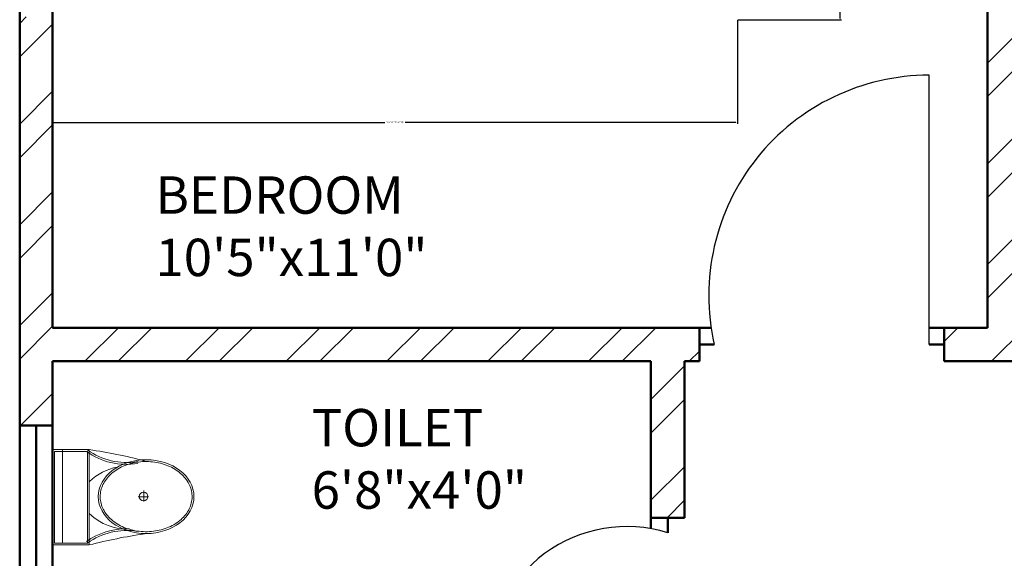
# Model space of a CAD drawing. Units: inches. Extents: x 1901 to 2863, y 888 to 2433.
# Tile 15 of 91: x 2025 to 2157, y 1549 to 1621. Entities that reach past the tile are written whole.
import ezdxf

# ---------------------------------------------------------------- set-up
doc = ezdxf.new("R2010")
doc.units = ezdxf.units.IN
for name, color, linetype, lineweight in [('A-ANNO-DIMS', 2, 'Continuous', 18), ('A-AREA-IDEN', 7, 'Continuous', 18), ('A-DOOR', 4, 'Continuous', 25), ('A-FLOR-FIXT', 9, 'Continuous', 18), ('A-WALL', 7, 'Continuous', 50), ('A-WALL-PATT', 8, 'Continuous', 13)]:
    doc.layers.add(name, color=color, linetype=linetype, lineweight=lineweight)
doc.styles.get("Standard").update_dxf_attribs({"font": 'arial.ttf'})
doc.dimstyles.get("Standard").update_dxf_attribs({"dimtxt": 0.18, "dimasz": 0.18, "dimexe": 0.18, "dimexo": 0.0625, "dimgap": 0.09, "dimtad": 0, "dimtih": 1, "dimtoh": 1, "dimdec": 4, "dimzin": 0, "dimdsep": 46, "dimtxsty": 'Standard', "dimcen": 0.09, "dimadec": 0, "dimazin": 0, "dimtfac": 1, "dimtdec": 4, "dimtofl": 0, "dimtmove": 0, "dimatfit": 3, "dimfxl": 1, "dimtolj": 1, "dimtzin": 0, "dimarcsym": 0})

# ---------------------------------------------------------------- blocks, each defined once
blk = doc.blocks.new('A$C31115884')
for p, q in [((283.1, 497.7), (223.4, 497.7)), ((257.5, 466.4), (257.5, 523.2)), ((0, 200), (0, 0)), ((520, 200), (0, 200)), ((10, 190), (10, 10)), ((510, 190), (10, 190)), ((510, 10), (510, 190)), ((520, 0), (520, 200)), ((510, 54.5), (0, 54.5)), ((10, 10), (510, 10)), ((0, 0), (520, 0))]:
    blk.add_line(p, q)
blk.add_circle((255.6, 496.4), 23.6)
for centre, radius, start, end in [((2777.7, -204.6), 2807, 165.4549, 171.7133), ((3237, 905), 2807, 188.2867, 194.5451), ((-294.5, 403.3), 364.7, 324.2091, 9.3499), ((-294.5, 403.3), 374.7, 324.2091, 9.3499), ((805.8, 403.3), 364.7, 170.6501, 215.7909), ((139.5, 406.2), 293.5, 315.8436, 2.6563), ((805.8, 403.3), 374.7, 179.2036, 215.7909), ((383.6, 406.2), 293.5, 190.2774, 224.1564)]:
    blk.add_arc(centre, radius, start, end)
blk.add_ellipse((256.2, 509.9), major_axis=(0, -260.7), ratio=0.772727)
blk.add_open_spline([(256.2, 259.2), (263.1, 259.2), (270, 259.7), (287.8, 262.3), (298.7, 265.1), (319.9, 273.1), (330.2, 278.4), (350.1, 291.1), (359.7, 298.7), (377.7, 315.9), (386.2, 325.5), (401.7, 346.6), (408.8, 358.1), (421.3, 382.5), (426.8, 395.5), (435.9, 422.4), (439.5, 436.4), (444.8, 465.1), (446.5, 479.7), (447.9, 509.2), (447.6, 524), (445, 553.3), (442.7, 567.8), (436.3, 596), (432.1, 609.7), (421.9, 636), (416, 648.6), (402.5, 672.1), (395, 683), (378.6, 703), (369.8, 712.1), (351.1, 728), (341.3, 734.8), (320.9, 746.2), (310.4, 750.7), (288.9, 757.3), (278, 759.4), (256, 761), (245, 760.6), (223.1, 757.2), (212.3, 754.3), (191.1, 746.1), (180.8, 740.7), (160.9, 727.8), (151.4, 720.1), (133.5, 702.7), (125.1, 693), (109.6, 671.7), (102.6, 660.2), (90.2, 635.7), (84.9, 622.7), (76, 595.6), (72.4, 581.6), (67.2, 552.9), (65.6, 538.2), (64.4, 508.8), (64.8, 494), (67.5, 464.7), (69.9, 450.2), (76.6, 422), (80.8, 408.3), (91.1, 382.2), (97.2, 369.7), (110.8, 346.3), (118.4, 335.4), (134.8, 315.6), (143.7, 306.7), (162.4, 290.9), (172.3, 284.2), (192.8, 273), (203.3, 268.6), (224.8, 262.2), (235.8, 260.2), (249.9, 259.3), (253, 259.2), (256.2, 259.2)], degree=3, knots=[0, 0, 0, 0, 0.110105, 0.110105, 0.285049, 0.285049, 0.459994, 0.459994, 0.634938, 0.634938, 0.809882, 0.809882, 0.984827, 0.984827, 1.159771, 1.159771, 1.334715, 1.334715, 1.50966, 1.50966, 1.684604, 1.684604, 1.859549, 1.859549, 2.034493, 2.034493, 2.209437, 2.209437, 2.384382, 2.384382, 2.559326, 2.559326, 2.73427, 2.73427, 2.909215, 2.909215, 3.084159, 3.084159, 3.259103, 3.259103, 3.434048, 3.434048, 3.608992, 3.608992, 3.783936, 3.783936, 3.958881, 3.958881, 4.133825, 4.133825, 4.30877, 4.30877, 4.483714, 4.483714, 4.658658, 4.658658, 4.833603, 4.833603, 5.008547, 5.008547, 5.183491, 5.183491, 5.358436, 5.358436, 5.53338, 5.53338, 5.708324, 5.708324, 5.883269, 5.883269, 6.058213, 6.058213, 6.233158, 6.233158, 6.283185, 6.283185, 6.283185, 6.283185])
blk = doc.blocks.new('*D17')
at = {"layer": 'A-ANNO-DIMS', "color": 0, "lineweight": -2, "transparency": 16777216}
for p, q in [((2029.33, 1621.25), (2029.33, 1607.4)), ((2120.88, 1621.25), (2120.88, 1607.4)), ((2029.51, 1607.58), (2073.74, 1607.58)), ((2120.7, 1607.58), (2076.47, 1607.58))]:
    blk.add_line(p, q, dxfattribs=at)
at = {"layer": 'A-ANNO-DIMS', "color": 0, "transparency": 16777216}
for points in [[(2029.51, 1607.61), (2029.51, 1607.55), (2029.33, 1607.58)], [(2120.7, 1607.61), (2120.7, 1607.55), (2120.88, 1607.58)]]:
    blk.add_solid(points, dxfattribs=at)
at = {"layer": 'Defpoints', "color": 0, "transparency": 16777216}
for p in [(2029.33, 1621.31), (2120.88, 1621.31), (2120.88, 1607.58)]:
    blk.add_point(p, dxfattribs=at)
at = {"layer": 'A-ANNO-DIMS', "color": 0, "transparency": 16777216, "insert": (2075.11, 1607.58), "char_height": 0.18, "attachment_point": 5}
blk.add_mtext('\\A1;DOUBLE BED 92 TYP.', dxfattribs=at)
blk = doc.blocks.new('*D18')
at = {"layer": 'A-ANNO-DIMS', "color": 0, "lineweight": -2, "transparency": 16777216}
for p, q in [((2120.95, 1683.99), (2134.8, 1683.99)), ((2134.62, 1683.81), (2134.62, 1652.83)), ((2134.62, 1621.49), (2134.62, 1652.47)), ((2120.95, 1621.31), (2134.8, 1621.31))]:
    blk.add_line(p, q, dxfattribs=at)
at = {"layer": 'A-ANNO-DIMS', "color": 0, "transparency": 16777216}
for points in [[(2134.59, 1683.81), (2134.65, 1683.81), (2134.62, 1683.99)], [(2134.59, 1621.49), (2134.65, 1621.49), (2134.62, 1621.31)]]:
    blk.add_solid(points, dxfattribs=at)
at = {"layer": 'Defpoints', "color": 0, "transparency": 16777216}
for p in [(2120.88, 1683.99), (2134.62, 1683.99), (2120.88, 1621.31)]:
    blk.add_point(p, dxfattribs=at)
at = {"layer": 'A-ANNO-DIMS', "color": 0, "transparency": 16777216, "insert": (2134.62, 1652.65), "char_height": 0.18, "attachment_point": 5}
blk.add_mtext('\\A1;63 TYP.', dxfattribs=at)

msp = doc.modelspace()

# ---------------------------------------------------------------- hatches: boundary and pattern name
at = {"layer": 'A-WALL-PATT'}
h = msp.add_hatch(dxfattribs=at)
h.set_pattern_fill('ANSI32', color=256)
h.paths.add_polyline_path([(2192.5, 2274.13), (2141.26, 2274.13), (2141.26, 2269.63), (2192.5, 2269.63)])
h.paths.add_polyline_path([(2259.93, 2274.13), (2216.5, 2274.13), (2216.5, 2269.63), (2255.43, 2269.63), (2255.43, 2214.63), (2250.81, 2214.63), (2250.81, 2210.13), (2259.93, 2210.13), (2259.93, 2215.13), (2271.76, 2215.13), (2271.76, 2217.38), (2271.76, 2219.63), (2259.93, 2219.63)])
h.paths.add_polyline_path([(2171.43, 2269.63), (2166.93, 2269.63), (2166.93, 2219.63), (2121.24, 2219.63), (2121.24, 2215.13), (2166.93, 2215.13), (2166.93, 2083.13), (2161.81, 2083.13), (2161.81, 2078.63), (2171.43, 2078.63), (2177, 2078.63), (2177, 2080.88), (2177, 2083.13), (2171.43, 2083.13), (2171.43, 2210.13), (2230.91, 2210.13), (2230.91, 2212.38), (2230.91, 2214.63), (2171.43, 2214.63)])
h.paths.add_polyline_path([(2117.26, 2274.13), (2089.43, 2274.13), (2089.43, 2219.63), (2081.14, 2219.63), (2081.14, 2215.13), (2089.43, 2215.13), (2098, 2215.13), (2098, 2217.38), (2098, 2219.63), (2093.93, 2219.63), (2093.93, 2269.63), (2117.26, 2269.63), (2117.26, 2271.88)])
h.paths.add_polyline_path([(2343.43, 2219.63), (2329.29, 2219.63), (2329.29, 2215.13), (2338.93, 2215.13), (2338.93, 2184.74), (2343.43, 2184.74)])
h.paths.add_polyline_path([(2338.93, 2083.13), (2329.29, 2083.13), (2208.97, 2083.13), (2208.97, 2078.63), (2338.93, 2078.63)])
h.paths.add_polyline_path([(2343.43, 2136.74), (2338.93, 2136.74), (2338.93, 1872.63), (2343.43, 1872.63)])
h.paths.add_polyline_path([(2343.43, 1863.63), (2397.68, 1863.63), (2397.68, 1821.63), (2384.14, 1821.63), (2384.14, 1812.63), (2418.33, 1812.63), (2418.33, 1817.13), (2418.33, 1821.63), (2406.68, 1821.63), (2406.68, 1863.63), (2459.5, 1863.63), (2459.5, 1821.63), (2447.14, 1821.63), (2447.14, 1812.63), (2459.5, 1812.63), (2468.5, 1812.63), (2468.5, 1872.63), (2394.43, 1872.63), (2334.43, 1872.63), (2334.43, 1812.63), (2343.43, 1812.63), (2353.25, 1812.63), (2353.25, 1821.63), (2343.43, 1821.63)])
h.paths.add_polyline_path([(2510.01, 1872.63), (2468.5, 1872.63), (2468.5, 1868.13), (2510.01, 1868.13)])
h.paths.add_polyline_path([(2514.01, 1817.13), (2468.5, 1817.13), (2468.5, 1812.63), (2482.11, 1812.63), (2482.11, 1800.61), (2486.61, 1800.61), (2486.61, 1812.63), (2514.01, 1812.63)])
h.paths.add_polyline_path([(2299.25, 1814.88), (2299.25, 1817.13), (2295.93, 1817.13), (2295.93, 1854.17), (2293.68, 1854.17), (2291.43, 1854.17), (2291.43, 1817.13), (2266.11, 1817.13), (2266.11, 1812.63), (2299.25, 1812.63)])
h.paths.add_polyline_path([(2218.11, 1817.13), (2206.46, 1817.13), (2171.43, 1817.13), (2171.43, 1949.13), (2190.1, 1949.13), (2190.1, 1953.63), (2163.47, 1953.63), (2163.47, 1949.13), (2166.93, 1949.13), (2166.93, 1817.13), (2114.3, 1817.13), (2114.3, 1812.63), (2218.11, 1812.63)])
h.paths.add_polyline_path([(2029.43, 1970.92), (2024.93, 1970.92), (2024.93, 1912.72), (2029.43, 1912.72)])
h.paths.add_polyline_path([(2132.3, 1953.63), (2113.93, 1953.63), (2113.93, 1975.89), (2111.68, 1975.89), (2109.43, 1975.89), (2109.43, 1953.63), (2029.43, 1953.63), (2029.43, 1949.13), (2132.3, 1949.13)])
h.paths.add_polyline_path([(2029.43, 1853.61), (2029.31, 1853.61), (2029.31, 1853.61), (2029.43, 1853.61), (2029.43, 1864.72), (2024.93, 1864.72), (2024.93, 1812.63), (2066.3, 1812.63), (2066.3, 1814.88), (2066.3, 1817.13), (2029.43, 1817.13)])
h.paths.add_polyline_path([(2122.93, 2010.09), (2120.68, 2010.09), (2118.43, 2010.09), (2118.43, 2006.13), (2029.43, 2006.13), (2029.43, 2001.63), (2109.43, 2001.63), (2109.43, 1998.04), (2113.93, 1998.04), (2113.93, 2001.63), (2122.93, 2001.63)])
h.paths.add_polyline_path([(2029.43, 2031.38), (2024.93, 2031.38), (2024.93, 1994.92), (2027.18, 1994.92), (2029.43, 1994.92)])
h.paths.add_polyline_path([(2029.43, 2136.74), (2024.93, 2136.74), (2024.93, 2067.38), (2027.18, 2067.38), (2029.43, 2067.38)])
h.paths.add_polyline_path([(2125.62, 2083.13), (2029.43, 2083.13), (2029.43, 2078.63), (2118.43, 2078.63), (2118.43, 2030.71), (2122.93, 2030.71), (2122.93, 2078.63), (2125.62, 2078.63)])
h.paths.add_polyline_path([(2029.43, 2215.13), (2040.47, 2215.13), (2040.47, 2217.38), (2040.47, 2219.63), (2024.93, 2219.63), (2024.93, 2184.74), (2029.43, 2184.74), (2029.43, 2187.78)])
h.paths.add_polyline_path([(2686.43, 2274.13), (2659.28, 2274.13), (2659.28, 2269.63), (2681.93, 2269.63), (2681.93, 2219.63), (2676.82, 2219.63), (2676.82, 2215.13), (2681.93, 2215.13), (2697.01, 2215.13), (2697.01, 2217.38), (2697.01, 2219.63), (2686.43, 2219.63)])
h.paths.add_polyline_path([(2609.93, 2269.63), (2635.28, 2269.63), (2635.28, 2274.13), (2571.43, 2274.13), (2571.43, 2269.63), (2605.43, 2269.63), (2605.43, 2214.63), (2549.1, 2214.63), (2549.1, 2210.13), (2605.43, 2210.13), (2605.43, 2083.13), (2601.01, 2083.13), (2601.01, 2080.88), (2601.01, 2078.63), (2609.93, 2078.63), (2616.16, 2078.63), (2616.16, 2080.88), (2616.16, 2083.13), (2609.93, 2083.13), (2609.93, 2215.13), (2651.46, 2215.13), (2651.46, 2217.38), (2651.46, 2219.63), (2609.93, 2219.63)])
h.paths.add_polyline_path([(2521.43, 2269.63), (2547.43, 2269.63), (2547.43, 2271.88), (2547.43, 2274.13), (2516.93, 2274.13), (2516.93, 2219.63), (2506.41, 2219.63), (2506.41, 2215.13), (2516.93, 2215.13), (2516.93, 2210.13), (2525.4, 2210.13), (2525.4, 2212.38), (2525.4, 2214.63), (2521.43, 2214.63)])
h.paths.add_polyline_path([(2456.01, 2219.63), (2439.43, 2219.63), (2439.43, 2187.89), (2443.93, 2187.89), (2443.93, 2215.13), (2456.01, 2215.13)])
h.paths.add_polyline_path([(2752.93, 2219.63), (2739.48, 2219.63), (2739.48, 2215.13), (2748.43, 2215.13), (2748.43, 2187.89), (2752.93, 2187.89)])
h.paths.add_polyline_path([(2752.93, 2139.89), (2748.43, 2139.89), (2748.43, 2083.13), (2648.42, 2083.13), (2648.42, 2078.63), (2654.93, 2078.63), (2654.93, 2039.44), (2659.43, 2039.44), (2659.43, 2078.63), (2748.43, 2078.63), (2748.43, 2063.43), (2752.93, 2063.43)])
h.paths.add_polyline_path([(2752.93, 2010.63), (2659.43, 2010.63), (2659.43, 2015.65), (2654.93, 2015.65), (2654.93, 2010.63), (2605.43, 2010.63), (2605.43, 1920.97), (2609.93, 1920.97), (2609.93, 2006.13), (2748.43, 2006.13), (2748.43, 1982.47), (2752.93, 1982.47)])
h.paths.add_polyline_path([(2752.93, 2027.43), (2748.43, 2027.43), (2748.43, 2010.63), (2752.93, 2010.63)])
h.paths.add_polyline_path([(2748.43, 1886.13), (2609.93, 1886.13), (2609.93, 1889.72), (2605.43, 1889.72), (2605.43, 1861.26), (2609.93, 1861.26), (2609.93, 1881.63), (2748.43, 1881.63)])
h.paths.add_polyline_path([(2456.86, 2228.83), (2498.4, 2228.83), (2498.4, 2247.49), (2456.86, 2247.49)], flags=9)
h.paths.add_polyline_path([(2038.6, 2237.42), (2080.17, 2237.42), (2080.17, 2256.08), (2038.6, 2256.08)], flags=9)
h.paths.add_polyline_path([(2292.01, 1062.39), (2539.93, 1062.39), (2539.93, 1099.49), (2292.01, 1099.49)], flags=9)
h.paths.add_polyline_path([(2424.91, 1832.25), (2448.51, 1832.25), (2448.51, 1846.68), (2424.91, 1846.68)], flags=25)
h.paths.add_polyline_path([(2359.08, 1832.25), (2382.68, 1832.25), (2382.68, 1846.68), (2359.08, 1846.68)], flags=25)
h.paths.add_polyline_path([(2352.9, 1684.8), (2367.54, 1684.8), (2367.54, 1697.17), (2352.9, 1697.17)], flags=9)
h.paths.add_polyline_path([(2079.29, 1755.83), (2169.02, 1755.83), (2169.02, 1774.37), (2079.29, 1774.37)], flags=9)
h.paths.add_polyline_path([(2404.09, 1373.86), (2404.09, 1463.59), (2385.54, 1463.59), (2385.54, 1373.86)], flags=9)
h.paths.add_polyline_path([(2268.09, 2236.37), (2309.64, 2236.37), (2309.64, 2255.03), (2268.09, 2255.03)], flags=9)
h.paths.add_polyline_path([(2575.96, 1700.95), (2665.7, 1700.95), (2665.7, 1719.5), (2575.96, 1719.5)], flags=9)
h.paths.add_polyline_path([(2302.96, 1878.47), (2329.52, 1878.47), (2329.52, 1888.78), (2302.96, 1888.78)], flags=9)
h.paths.add_polyline_path([(2097.42, 2240.58), (2126.57, 2240.58), (2126.57, 2259.23), (2097.42, 2259.23)], flags=9)
h.paths.add_polyline_path([(2208.72, 2246.12), (2237.88, 2246.12), (2237.88, 2264.78), (2208.72, 2264.78)], flags=9)
h.paths.add_polyline_path([(2038.15, 1925.96), (2076.99, 1925.96), (2076.99, 1944.62), (2038.15, 1944.62)], flags=9)
h.paths.add_polyline_path([(2239.14, 1926.67), (2288.46, 1926.67), (2288.46, 1945.33), (2239.14, 1945.33)], flags=9)
h.paths.add_polyline_path([(2175.43, 2007.33), (2212.36, 2007.33), (2212.36, 2025.99), (2175.43, 2025.99)], flags=9)
h.paths.add_polyline_path([(2225.03, 2091.79), (2263.87, 2091.79), (2263.87, 2110.45), (2225.03, 2110.45)], flags=9)
h.paths.add_polyline_path([(2035.4, 2098.48), (2074.24, 2098.48), (2074.24, 2117.14), (2035.4, 2117.14)], flags=9)
h.paths.add_polyline_path([(2050.1, 2029.21), (2083.26, 2029.21), (2083.26, 2047.87), (2050.1, 2047.87)], flags=9)
h.paths.add_polyline_path([(2069.68, 1956.72), (2098.83, 1956.72), (2098.83, 1975.38), (2069.68, 1975.38)], flags=25)
h.paths.add_polyline_path([(2328.62, 1753.34), (2361.66, 1753.34), (2361.66, 1771.99), (2328.62, 1771.99)], flags=9)
h.paths.add_polyline_path([(2395.16, 2060.89), (2395.16, 2140.65), (2378.68, 2140.65), (2378.68, 2060.89)], flags=9)
h.paths.add_polyline_path([(2463.73, 2059.02), (2492.89, 2059.02), (2492.89, 2077.68), (2463.73, 2077.68)], flags=9)
h.paths.add_polyline_path([(2458.03, 2181.54), (2496.87, 2181.54), (2496.87, 2200.19), (2458.03, 2200.19)], flags=9)
h.paths.add_polyline_path([(2527.58, 2243.07), (2556.73, 2243.07), (2556.73, 2261.73), (2527.58, 2261.73)], flags=9)
h.paths.add_polyline_path([(2694.46, 2232.77), (2736.03, 2232.77), (2736.03, 2251.42), (2694.46, 2251.42)], flags=9)
h.paths.add_polyline_path([(2637.82, 2249.22), (2666.98, 2249.22), (2666.98, 2267.88), (2637.82, 2267.88)], flags=9)
h.paths.add_polyline_path([(2623.69, 2183.54), (2662.53, 2183.54), (2662.53, 2202.2), (2623.69, 2202.2)], flags=9)
h.paths.add_polyline_path([(2691.97, 2021.5), (2725.12, 2021.5), (2725.12, 2040.16), (2691.97, 2040.16)], flags=9)
h.paths.add_polyline_path([(2621.04, 1975.91), (2662.34, 1975.91), (2662.34, 1994.57), (2621.04, 1994.57)], flags=25)
h.paths.add_polyline_path([(2479.03, 1927.62), (2519.84, 1927.62), (2519.84, 1946.28), (2479.03, 1946.28)], flags=9)
h.paths.add_polyline_path([(2670.94, 1849.08), (2716.01, 1849.08), (2716.01, 1867.73), (2670.94, 1867.73)], flags=9)
h.paths.add_polyline_path([(2523.61, 1782.96), (2550.17, 1782.96), (2550.17, 1793.26), (2523.61, 1793.26)], flags=9)
h.paths.add_polyline_path([(2450.84, 1207.33), (2492.39, 1207.33), (2492.39, 1225.99), (2450.84, 1225.99)], flags=9)
h.paths.add_polyline_path([(2527.75, 1203.84), (2556.91, 1203.84), (2556.91, 1222.5), (2527.75, 1222.5)], flags=9)
h.paths.add_polyline_path([(2639.11, 1207.2), (2668.27, 1207.2), (2668.27, 1225.86), (2639.11, 1225.86)], flags=9)
h.paths.add_polyline_path([(2692.59, 1218.97), (2734.17, 1218.97), (2734.17, 1237.62), (2692.59, 1237.62)], flags=9)
h.paths.add_polyline_path([(2669.27, 1366.33), (2708.11, 1366.33), (2708.11, 1384.99), (2669.27, 1384.99)], flags=9)
h.paths.add_polyline_path([(2463.31, 1358.03), (2502.15, 1358.03), (2502.15, 1376.69), (2463.31, 1376.69)], flags=9)
h.paths.add_polyline_path([(2494.72, 1449.96), (2531.65, 1449.96), (2531.65, 1468.62), (2494.72, 1468.62)], flags=9)
h.paths.add_polyline_path([(2675.57, 1422.16), (2708.72, 1422.16), (2708.72, 1440.81), (2675.57, 1440.81)], flags=9)
h.paths.add_polyline_path([(2685.63, 1493.89), (2714.79, 1493.89), (2714.79, 1512.55), (2685.63, 1512.55)], flags=9)
h.paths.add_polyline_path([(2686.8, 1529.91), (2725.65, 1529.91), (2725.65, 1548.57), (2686.8, 1548.57)], flags=9)
h.paths.add_polyline_path([(2503.65, 1537.99), (2552.97, 1537.99), (2552.97, 1556.65), (2503.65, 1556.65)], flags=9)
h.paths.add_polyline_path([(2291.71, 1643.5), (2318.28, 1643.5), (2318.28, 1653.81), (2291.71, 1653.81)], flags=9)
h.paths.add_polyline_path([(2450.63, 1610.52), (2477.19, 1610.52), (2477.19, 1620.82), (2450.63, 1620.82)], flags=9)
h.paths.add_polyline_path([(2359.99, 1551.81), (2422.25, 1551.81), (2422.25, 1562.12), (2359.99, 1562.12)], flags=9)
h.paths.add_polyline_path([(2280.11, 1249.01), (2321.65, 1249.01), (2321.65, 1267.66), (2280.11, 1267.66)], flags=9)
h.paths.add_polyline_path([(2164.06, 1274.23), (2193.22, 1274.23), (2193.22, 1292.89), (2164.06, 1292.89)], flags=9)
h.paths.add_polyline_path([(2118.21, 1277.69), (2151.25, 1277.69), (2151.25, 1296.35), (2118.21, 1296.35)], flags=9)
h.paths.add_polyline_path([(2031.95, 1268.53), (2073.52, 1268.53), (2073.52, 1287.19), (2031.95, 1287.19)], flags=9)
h.paths.add_polyline_path([(2050.2, 1409.08), (2089.04, 1409.08), (2089.04, 1427.74), (2050.2, 1427.74)], flags=9)
h.paths.add_polyline_path([(2243.74, 1421.03), (2282.58, 1421.03), (2282.58, 1439.69), (2243.74, 1439.69)], flags=9)
h.paths.add_polyline_path([(2190.75, 1509.77), (2231.56, 1509.77), (2231.56, 1528.43), (2190.75, 1528.43)], flags=9)
h.paths.add_polyline_path([(2058.39, 1475.42), (2091.55, 1475.42), (2091.55, 1494.07), (2058.39, 1494.07)], flags=9)
h.paths.add_polyline_path([(2062.45, 1553.09), (2091.6, 1553.09), (2091.6, 1571.75), (2062.45, 1571.75)], flags=9)
h.paths.add_polyline_path([(2219.52, 1590.37), (2266.15, 1590.37), (2266.15, 1609.02), (2219.52, 1609.02)], flags=9)
h.paths.add_polyline_path([(2041.07, 1584.19), (2079.91, 1584.19), (2079.91, 1602.85), (2041.07, 1602.85)], flags=9)
h = msp.add_hatch(dxfattribs=at)
h.set_pattern_fill('ANSI32', color=256)
h.paths.add_polyline_path([(2443.93, 2139.89), (2439.43, 2139.89), (2439.43, 2069.35), (2441.68, 2069.35), (2443.93, 2069.35), (2443.93, 2078.63), (2521.93, 2078.63), (2521.93, 2075.07), (2524.18, 2075.07), (2526.43, 2075.07), (2526.43, 2078.63), (2571.75, 2078.63), (2571.75, 2080.88), (2571.75, 2083.13), (2443.93, 2083.13)])
h.paths.add_polyline_path([(2526.43, 2054.63), (2524.18, 2054.63), (2521.93, 2054.63), (2521.93, 2030.63), (2443.93, 2030.63), (2443.93, 2045.35), (2439.43, 2045.35), (2439.43, 1983.87), (2443.93, 1983.87), (2443.93, 2026.13), (2521.93, 2026.13), (2526.43, 2026.13)])
h.paths.add_polyline_path([(2443.93, 1923.87), (2439.43, 1923.87), (2439.43, 1872.63), (2443.93, 1872.63)])
h.paths.add_polyline_path([(2636.23, 1766.13), (2609.93, 1766.13), (2609.93, 1779.79), (2605.43, 1779.79), (2605.43, 1766.13), (2486.61, 1766.13), (2486.61, 1770.67), (2482.11, 1770.67), (2482.11, 1766.13), (2482.11, 1761.63), (2636.23, 1761.63), (2636.23, 1763.88)])
h.paths.add_polyline_path([(2519.54, 1663.38), (2519.54, 1665.63), (2494.93, 1665.63), (2481.83, 1665.63), (2481.83, 1663.38), (2481.83, 1661.13), (2490.43, 1661.13), (2490.43, 1640.16), (2494.93, 1640.16), (2494.93, 1661.13), (2519.54, 1661.13)])
h.paths.add_polyline_path([(2443.93, 1712.13), (2443.93, 1716.63), (2414.46, 1716.63), (2414.46, 1712.13), (2439.43, 1712.13), (2439.43, 1545.51), (2443.93, 1545.51), (2443.93, 1661.13), (2448.47, 1661.13), (2448.47, 1665.63), (2443.93, 1665.63)])
h.paths.add_polyline_path([(2343.43, 1712.13), (2365.52, 1712.13), (2365.52, 1714.38), (2365.52, 1716.63), (2333.87, 1716.63), (2333.87, 1714.38), (2333.87, 1712.13), (2338.93, 1712.13), (2338.93, 1575.63), (2338.93, 1545.51), (2343.43, 1545.51), (2343.43, 1547.51), (2343.43, 1580.13)])
h.paths.add_polyline_path([(2752.93, 1665.63), (2579.54, 1665.63), (2579.54, 1661.13), (2615.93, 1661.13), (2615.93, 1529.13), (2598.93, 1529.13), (2598.93, 1524.63), (2623.13, 1524.63), (2623.13, 1526.88), (2623.13, 1529.13), (2620.43, 1529.13), (2620.43, 1661.13), (2748.43, 1661.13), (2748.43, 1633.5), (2752.93, 1633.5)])
h.paths.add_polyline_path([(2752.93, 1419.93), (2748.43, 1419.93), (2748.43, 1400.13), (2659.43, 1400.13), (2659.43, 1444.33), (2657.18, 1444.33), (2654.93, 1444.33), (2654.93, 1400.13), (2643.65, 1400.13), (2643.65, 1395.63), (2748.43, 1395.63), (2748.43, 1364.04), (2752.93, 1364.04)])
h.paths.add_polyline_path([(2752.93, 1492.88), (2748.43, 1492.88), (2748.43, 1476.63), (2667.43, 1476.63), (2667.43, 1479.71), (2665.18, 1479.71), (2662.93, 1479.71), (2662.93, 1476.63), (2654.93, 1476.63), (2654.93, 1469.54), (2659.43, 1469.54), (2659.43, 1472.13), (2748.43, 1472.13), (2748.43, 1455.93), (2752.93, 1455.93)])
h.paths.add_polyline_path([(2752.93, 1304.04), (2748.43, 1304.04), (2748.43, 1263.63), (2738.66, 1263.63), (2738.66, 1259.13), (2752.93, 1259.13)])
h.paths.add_polyline_path([(2685.93, 1259.13), (2695.49, 1259.13), (2695.49, 1261.38), (2695.49, 1263.63), (2677.84, 1263.63), (2677.84, 1261.38), (2677.84, 1259.13), (2681.43, 1259.13), (2681.43, 1203.63), (2653.28, 1203.63), (2653.28, 1199.13), (2685.93, 1199.13), (2685.93, 1203.63)])
h.paths.add_polyline_path([(2609.43, 1395.63), (2611.85, 1395.63), (2611.85, 1400.13), (2598.89, 1400.13), (2598.89, 1397.88), (2598.89, 1395.63), (2604.93, 1395.63), (2604.93, 1268.13), (2554.73, 1268.13), (2554.73, 1265.88), (2554.73, 1263.63), (2604.93, 1263.63), (2604.93, 1203.63), (2571.31, 1203.63), (2571.31, 1199.13), (2604.93, 1199.13), (2629.28, 1199.13), (2629.28, 1201.38), (2629.28, 1203.63), (2609.43, 1203.63), (2609.43, 1258.63), (2609.43, 1259.13), (2654.8, 1259.13), (2654.8, 1263.63), (2609.43, 1263.63)])
h.paths.add_polyline_path([(2443.93, 1304.04), (2439.43, 1304.04), (2439.43, 1259.13), (2443.93, 1259.13), (2456.16, 1259.13), (2456.16, 1261.38), (2456.16, 1263.63), (2443.93, 1263.63)])
h.paths.add_polyline_path([(2525.43, 1263.63), (2531.78, 1263.63), (2531.78, 1268.13), (2520.93, 1268.13), (2520.93, 1263.63), (2511.41, 1263.63), (2511.41, 1259.13), (2520.93, 1259.13), (2520.93, 1199.13), (2547.31, 1199.13), (2547.31, 1201.38), (2547.31, 1203.63), (2525.43, 1203.63)])
h.paths.add_polyline_path([(2443.93, 1434.84), (2439.43, 1434.84), (2439.43, 1364.04), (2441.68, 1364.04), (2443.93, 1364.04)])
h.paths.add_polyline_path([(2567.13, 1400.13), (2443.93, 1400.13), (2443.93, 1395.63), (2567.13, 1395.63)])
h.paths.add_polyline_path([(2443.93, 1545.51), (2439.43, 1545.51), (2439.43, 1494.84), (2443.93, 1494.84)])
h.paths.add_polyline_path([(2494.93, 1553.35), (2492.68, 1553.35), (2490.43, 1553.35), (2490.43, 1524.63), (2494.93, 1524.63), (2525.94, 1524.63), (2525.94, 1526.88), (2525.94, 1529.13), (2494.93, 1529.13)])
h.paths.add_polyline_path([(2752.93, 1573.5), (2748.43, 1573.5), (2748.43, 1529.13), (2657.76, 1529.13), (2657.76, 1524.63), (2662.93, 1524.63), (2662.93, 1498.63), (2667.43, 1498.63), (2667.43, 1524.63), (2748.43, 1524.63), (2748.43, 1516.88), (2752.93, 1516.88)])
h.paths.add_polyline_path([(2038.6, 2237.42), (2080.17, 2237.42), (2080.17, 2256.08), (2038.6, 2256.08)], flags=9)
h.paths.add_polyline_path([(2292.01, 1062.39), (2539.93, 1062.39), (2539.93, 1099.49), (2292.01, 1099.49)], flags=9)
h.paths.add_polyline_path([(2424.91, 1832.25), (2448.51, 1832.25), (2448.51, 1846.68), (2424.91, 1846.68)], flags=9)
h.paths.add_polyline_path([(2359.08, 1832.25), (2382.68, 1832.25), (2382.68, 1846.68), (2359.08, 1846.68)], flags=9)
h.paths.add_polyline_path([(2352.9, 1684.8), (2367.54, 1684.8), (2367.54, 1697.17), (2352.9, 1697.17)], flags=9)
h.paths.add_polyline_path([(2079.29, 1755.83), (2169.02, 1755.83), (2169.02, 1774.37), (2079.29, 1774.37)], flags=9)
h.paths.add_polyline_path([(2404.09, 1373.86), (2404.09, 1463.59), (2385.54, 1463.59), (2385.54, 1373.86)], flags=9)
h.paths.add_polyline_path([(2268.09, 2236.37), (2309.64, 2236.37), (2309.64, 2255.03), (2268.09, 2255.03)], flags=9)
h.paths.add_polyline_path([(2575.96, 1700.95), (2665.7, 1700.95), (2665.7, 1719.5), (2575.96, 1719.5)], flags=9)
h.paths.add_polyline_path([(2302.96, 1878.47), (2329.52, 1878.47), (2329.52, 1888.78), (2302.96, 1888.78)], flags=9)
h.paths.add_polyline_path([(2097.42, 2240.58), (2126.57, 2240.58), (2126.57, 2259.23), (2097.42, 2259.23)], flags=9)
h.paths.add_polyline_path([(2208.72, 2246.12), (2237.88, 2246.12), (2237.88, 2264.78), (2208.72, 2264.78)], flags=9)
h.paths.add_polyline_path([(2038.15, 1925.96), (2076.99, 1925.96), (2076.99, 1944.62), (2038.15, 1944.62)], flags=9)
h.paths.add_polyline_path([(2239.14, 1926.67), (2288.46, 1926.67), (2288.46, 1945.33), (2239.14, 1945.33)], flags=9)
h.paths.add_polyline_path([(2175.43, 2007.33), (2212.36, 2007.33), (2212.36, 2025.99), (2175.43, 2025.99)], flags=9)
h.paths.add_polyline_path([(2225.03, 2091.79), (2263.87, 2091.79), (2263.87, 2110.45), (2225.03, 2110.45)], flags=9)
h.paths.add_polyline_path([(2035.4, 2098.48), (2074.24, 2098.48), (2074.24, 2117.14), (2035.4, 2117.14)], flags=9)
h.paths.add_polyline_path([(2050.1, 2029.21), (2083.26, 2029.21), (2083.26, 2047.87), (2050.1, 2047.87)], flags=9)
h.paths.add_polyline_path([(2069.68, 1956.72), (2098.83, 1956.72), (2098.83, 1975.38), (2069.68, 1975.38)], flags=9)
h.paths.add_polyline_path([(2328.62, 1753.34), (2361.66, 1753.34), (2361.66, 1771.99), (2328.62, 1771.99)], flags=9)
h.paths.add_polyline_path([(2395.16, 2060.89), (2395.16, 2140.65), (2378.68, 2140.65), (2378.68, 2060.89)], flags=9)
h.paths.add_polyline_path([(2463.73, 2059.02), (2492.89, 2059.02), (2492.89, 2077.68), (2463.73, 2077.68)], flags=9)
h.paths.add_polyline_path([(2458.03, 2181.54), (2496.87, 2181.54), (2496.87, 2200.19), (2458.03, 2200.19)], flags=9)
h.paths.add_polyline_path([(2456.86, 2228.83), (2498.4, 2228.83), (2498.4, 2247.49), (2456.86, 2247.49)], flags=9)
h.paths.add_polyline_path([(2527.58, 2243.07), (2556.73, 2243.07), (2556.73, 2261.73), (2527.58, 2261.73)], flags=9)
h.paths.add_polyline_path([(2694.46, 2232.77), (2736.03, 2232.77), (2736.03, 2251.42), (2694.46, 2251.42)], flags=9)
h.paths.add_polyline_path([(2637.82, 2249.22), (2666.98, 2249.22), (2666.98, 2267.88), (2637.82, 2267.88)], flags=9)
h.paths.add_polyline_path([(2623.69, 2183.54), (2662.53, 2183.54), (2662.53, 2202.2), (2623.69, 2202.2)], flags=9)
h.paths.add_polyline_path([(2691.97, 2021.5), (2725.12, 2021.5), (2725.12, 2040.16), (2691.97, 2040.16)], flags=9)
h.paths.add_polyline_path([(2621.04, 1975.91), (2662.34, 1975.91), (2662.34, 1994.57), (2621.04, 1994.57)], flags=9)
h.paths.add_polyline_path([(2479.03, 1927.62), (2519.84, 1927.62), (2519.84, 1946.28), (2479.03, 1946.28)], flags=9)
h.paths.add_polyline_path([(2670.94, 1849.08), (2716.01, 1849.08), (2716.01, 1867.73), (2670.94, 1867.73)], flags=9)
h.paths.add_polyline_path([(2523.61, 1782.96), (2550.17, 1782.96), (2550.17, 1793.26), (2523.61, 1793.26)], flags=9)
h.paths.add_polyline_path([(2450.84, 1207.33), (2492.39, 1207.33), (2492.39, 1225.99), (2450.84, 1225.99)], flags=9)
h.paths.add_polyline_path([(2527.75, 1203.84), (2556.91, 1203.84), (2556.91, 1222.5), (2527.75, 1222.5)], flags=9)
h.paths.add_polyline_path([(2639.11, 1207.2), (2668.27, 1207.2), (2668.27, 1225.86), (2639.11, 1225.86)], flags=9)
h.paths.add_polyline_path([(2692.59, 1218.97), (2734.17, 1218.97), (2734.17, 1237.62), (2692.59, 1237.62)], flags=9)
h.paths.add_polyline_path([(2669.27, 1366.33), (2708.11, 1366.33), (2708.11, 1384.99), (2669.27, 1384.99)], flags=25)
h.paths.add_polyline_path([(2463.31, 1358.03), (2502.15, 1358.03), (2502.15, 1376.69), (2463.31, 1376.69)], flags=9)
h.paths.add_polyline_path([(2494.72, 1449.96), (2531.65, 1449.96), (2531.65, 1468.62), (2494.72, 1468.62)], flags=9)
h.paths.add_polyline_path([(2675.57, 1422.16), (2708.72, 1422.16), (2708.72, 1440.81), (2675.57, 1440.81)], flags=25)
h.paths.add_polyline_path([(2685.63, 1493.89), (2714.79, 1493.89), (2714.79, 1512.55), (2685.63, 1512.55)], flags=9)
h.paths.add_polyline_path([(2686.8, 1529.91), (2725.65, 1529.91), (2725.65, 1548.57), (2686.8, 1548.57)], flags=25)
h.paths.add_polyline_path([(2503.65, 1537.99), (2552.97, 1537.99), (2552.97, 1556.65), (2503.65, 1556.65)], flags=9)
h.paths.add_polyline_path([(2291.71, 1643.5), (2318.28, 1643.5), (2318.28, 1653.81), (2291.71, 1653.81)], flags=9)
h.paths.add_polyline_path([(2450.63, 1610.52), (2477.19, 1610.52), (2477.19, 1620.82), (2450.63, 1620.82)], flags=9)
h.paths.add_polyline_path([(2359.99, 1551.81), (2422.25, 1551.81), (2422.25, 1562.12), (2359.99, 1562.12)], flags=9)
h.paths.add_polyline_path([(2280.11, 1249.01), (2321.65, 1249.01), (2321.65, 1267.66), (2280.11, 1267.66)], flags=9)
h.paths.add_polyline_path([(2164.06, 1274.23), (2193.22, 1274.23), (2193.22, 1292.89), (2164.06, 1292.89)], flags=9)
h.paths.add_polyline_path([(2118.21, 1277.69), (2151.25, 1277.69), (2151.25, 1296.35), (2118.21, 1296.35)], flags=9)
h.paths.add_polyline_path([(2031.95, 1268.53), (2073.52, 1268.53), (2073.52, 1287.19), (2031.95, 1287.19)], flags=9)
h.paths.add_polyline_path([(2050.2, 1409.08), (2089.04, 1409.08), (2089.04, 1427.74), (2050.2, 1427.74)], flags=9)
h.paths.add_polyline_path([(2243.74, 1421.03), (2282.58, 1421.03), (2282.58, 1439.69), (2243.74, 1439.69)], flags=9)
h.paths.add_polyline_path([(2190.75, 1509.77), (2231.56, 1509.77), (2231.56, 1528.43), (2190.75, 1528.43)], flags=9)
h.paths.add_polyline_path([(2058.39, 1475.42), (2091.55, 1475.42), (2091.55, 1494.07), (2058.39, 1494.07)], flags=9)
h.paths.add_polyline_path([(2062.45, 1553.09), (2091.6, 1553.09), (2091.6, 1571.75), (2062.45, 1571.75)], flags=9)
h.paths.add_polyline_path([(2219.52, 1590.37), (2266.15, 1590.37), (2266.15, 1609.02), (2219.52, 1609.02)], flags=9)
h.paths.add_polyline_path([(2041.07, 1584.19), (2079.91, 1584.19), (2079.91, 1602.85), (2041.07, 1602.85)], flags=9)
h = msp.add_hatch(dxfattribs=at)
h.set_pattern_fill('ANSI32', color=256)
h.paths.add_polyline_path([(2182.93, 1716.63), (2024.93, 1716.63), (2024.93, 1681.7), (2029.33, 1681.7), (2029.33, 1712.13), (2154.33, 1712.13), (2154.33, 1580.13), (2148.52, 1580.13), (2148.52, 1577.88), (2148.52, 1575.63), (2194.93, 1575.63), (2194.93, 1580.13), (2158.83, 1580.13), (2158.83, 1712.13), (2182.93, 1712.13)])
h.paths.add_polyline_path([(2301.07, 1716.63), (2242.93, 1716.63), (2242.93, 1712.13), (2283.83, 1712.13), (2283.83, 1685.54), (2288.33, 1685.54), (2288.33, 1712.13), (2301.07, 1712.13)])
h.paths.add_polyline_path([(2288.33, 1600.41), (2286.08, 1600.41), (2283.83, 1600.41), (2283.83, 1580.13), (2270.6, 1580.13), (2270.6, 1575.63), (2288.33, 1575.63)])
h.paths.add_polyline_path([(2295.93, 1953.63), (2271.45, 1953.63), (2271.45, 1949.13), (2291.43, 1949.13), (2291.43, 1941.24), (2295.93, 1941.24)])
h.paths.add_polyline_path([(2098.38, 1244.13), (2082.33, 1244.13), (2082.33, 1302.13), (2086.52, 1302.13), (2086.52, 1306.63), (2067.46, 1306.63), (2067.46, 1302.13), (2077.83, 1302.13), (2077.83, 1239.63), (2098.38, 1239.63), (2098.38, 1241.88)])
h.paths.add_polyline_path([(2217.31, 1306.63), (2158.83, 1306.63), (2158.83, 1451.63), (2162.72, 1451.63), (2162.72, 1453.88), (2162.72, 1456.13), (2154.33, 1456.13), (2154.33, 1443.13), (2151.91, 1443.13), (2151.91, 1438.63), (2154.33, 1438.63), (2154.33, 1306.63), (2109.31, 1306.63), (2109.31, 1304.38), (2109.31, 1302.13), (2154.33, 1302.13), (2154.33, 1244.13), (2122.38, 1244.13), (2122.38, 1239.63), (2154.33, 1239.63), (2154.33, 1223.63), (2163.33, 1223.63), (2181.01, 1223.63), (2181.01, 1225.88), (2181.01, 1228.13), (2163.33, 1228.13), (2163.33, 1258.22), (2158.83, 1258.22), (2158.83, 1302.13), (2217.31, 1302.13)])
h.paths.add_polyline_path([(2259.99, 1306.63), (2238.3, 1306.63), (2238.3, 1304.38), (2238.3, 1302.13), (2242.83, 1302.13), (2242.83, 1228.13), (2205.01, 1228.13), (2205.01, 1223.63), (2247.33, 1223.63), (2247.33, 1302.13), (2259.99, 1302.13), (2259.99, 1304.38)])
h.paths.add_polyline_path([(2343.43, 1361.7), (2338.93, 1361.7), (2338.93, 1306.63), (2322.38, 1306.63), (2322.38, 1302.13), (2343.43, 1302.13)])
h.paths.add_polyline_path([(2343.43, 1470.4), (2338.93, 1470.4), (2338.93, 1456.13), (2193.73, 1456.13), (2193.73, 1453.88), (2193.73, 1451.63), (2338.93, 1451.63), (2338.93, 1421.7), (2343.43, 1421.7)])
h.paths.add_polyline_path([(2343.43, 1545.51), (2338.93, 1545.51), (2338.93, 1530.4), (2343.43, 1530.4)])
h.paths.add_polyline_path([(2029.33, 1466.83), (2024.93, 1466.83), (2024.93, 1409.82), (2029.33, 1409.82)])
h.paths.add_polyline_path([(2122.84, 1440.88), (2122.84, 1443.13), (2121.83, 1443.13), (2121.83, 1498.18), (2119.58, 1498.18), (2117.33, 1498.18), (2117.33, 1443.13), (2029.33, 1443.13), (2029.33, 1438.63), (2122.84, 1438.63)])
h.paths.add_polyline_path([(2029.33, 1543.05), (2024.93, 1543.05), (2024.93, 1502.83), (2029.33, 1502.83)])
h.paths.add_polyline_path([(2029.33, 1621.7), (2024.93, 1621.7), (2024.93, 1567.05), (2027.13, 1567.05), (2029.33, 1567.05), (2029.33, 1575.63), (2109.33, 1575.63), (2109.33, 1554.71), (2113.83, 1554.71), (2113.83, 1575.63), (2115.8, 1575.63), (2115.8, 1577.88), (2115.8, 1580.13), (2029.33, 1580.13)])
h.paths.add_polyline_path([(2121.83, 1527.63), (2117.33, 1527.63), (2113.83, 1527.63), (2113.83, 1533.01), (2111.58, 1533.01), (2109.33, 1533.01), (2109.33, 1527.63), (2029.33, 1527.63), (2029.33, 1523.13), (2117.33, 1523.13), (2117.33, 1519.43), (2121.83, 1519.43)])
h.paths.add_polyline_path([(2029.33, 1349.82), (2024.93, 1349.82), (2024.93, 1302.13), (2036.28, 1302.13), (2036.28, 1306.63), (2029.33, 1306.63)])

# ---------------------------------------------------------------- linework, layer by layer
at = {"layer": 'A-DOOR'}
msp.add_line((2146.52, 1577.88), (2146.52, 1613.88), dxfattribs=at)
for centre, radius, start, end in [((2146.52, 1584.43), 29.46, 90, 192.8363), ((2106.11, 1535.01), 18.53, 72.8301, 180)]:
    msp.add_arc(centre, radius, start, end, dxfattribs=at)
at = {"layer": 'A-WALL'}
for p, q in [((2024.93, 1716.63), (2024.93, 1302.13)), ((2029.33, 1712.13), (2029.33, 1580.13)), ((2154.33, 1712.13), (2154.33, 1580.13)), ((2117.38, 1580.13), (2029.33, 1580.13)), ((2115.8, 1580.13), (2115.8, 1575.63)), ((2154.33, 1580.13), (2146.52, 1580.13)), ((2148.52, 1580.13), (2148.52, 1575.63)), ((2148.52, 1575.63), (2148.52, 1580.13)), ((2148.52, 1580.13), (2148.52, 1577.88)), ((2115.8, 1575.63), (2115.8, 1577.88)), ((2115.8, 1577.88), (2117.8, 1577.88)), ((2148.52, 1577.88), (2146.52, 1577.88)), ((2029.33, 1575.63), (2029.33, 1306.63)), ((2029.33, 1575.63), (2109.33, 1575.63)), ((2109.33, 1575.63), (2029.33, 1575.63)), ((2109.33, 1575.63), (2109.33, 1553.26)), ((2115.8, 1575.63), (2113.83, 1575.63)), ((2113.83, 1554.71), (2113.83, 1575.63)), ((2194.93, 1575.63), (2148.52, 1575.63)), ((2024.93, 1567.05), (2029.33, 1567.05)), ((2029.33, 1567.05), (2024.93, 1567.05)), ((2024.93, 1567.05), (2027.13, 1567.05)), ((2027.13, 1567.05), (2027.13, 1543.05)), ((2109.33, 1554.71), (2113.83, 1554.71)), ((2113.83, 1554.71), (2111.58, 1554.71)), ((2111.58, 1554.71), (2111.58, 1552.71))]:
    msp.add_line(p, q, dxfattribs=at)

# ---------------------------------------------------------------- block references
at = {"layer": 'A-FLOR-FIXT', "xscale": 0.0245149588751191, "yscale": 0.0245149588751191, "zscale": 0.0245149588751191, "rotation": 270}
msp.add_blockref('A$C31115884', (2029.33, 1563.82), dxfattribs=at)

# ---------------------------------------------------------------- texts
at = {"layer": 'A-AREA-IDEN', "char_height": 5, "attachment_point": 1}
for s, width, insert in [('BEDROOM\\P10\'5"x11\'0"', 166.4034, (2043.08, 1600.36)), ('TOILET\\P6\'8"x4\'0"', 78.2547, (2063.96, 1569.26))]:
    msp.add_mtext_dynamic_manual_height_columns(s, width=width, gutter_width=12.5, heights=[0], dxfattribs=dict(at, insert=insert))

# ---------------------------------------------------------------- dimensions: what is measured, and where the dimension line sits
at = {"layer": 'A-ANNO-DIMS'}
dim = msp.add_linear_dim(base=(2134.62, 1683.99), p1=(2120.88, 1621.31), p2=(2120.88, 1683.99), angle=90, text='<> TYP.', dimstyle='Standard', override={"dimdec": 0, "dimlfac": 1, "dimrnd": 0, "dimzin": 0, "dimdsep": 46, "dimlunit": 2}, dxfattribs=at)
dim.commit()
dim.dimension.update_dxf_attribs({"geometry": '*D18', "text_midpoint": (2134.62, 1652.65)})
dim = msp.add_linear_dim(base=(2120.88, 1607.58), p1=(2029.33, 1621.31), p2=(2120.88, 1621.31), text='DOUBLE BED <> TYP.', dimstyle='Standard', override={"dimdec": 0, "dimlfac": 1, "dimrnd": 0, "dimzin": 0, "dimdsep": 46, "dimlunit": 2}, dxfattribs=at)
dim.commit()
dim.dimension.update_dxf_attribs({"geometry": '*D17', "text_midpoint": (2075.11, 1607.58)})

doc.saveas('drawing.dxf')
